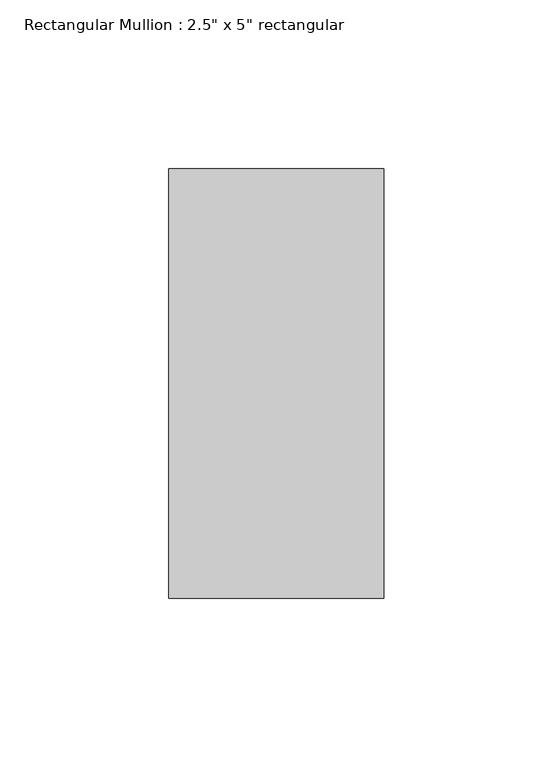
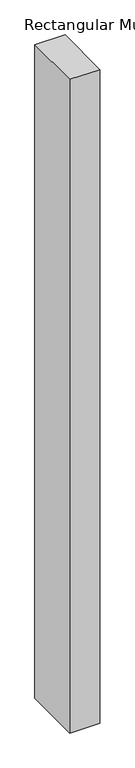
"""IFC4 building model written with IfcOpenShell, lengths in millimetres: member geometry."""

from ifc_helpers import new_model, si_unit, frame, origin, place, context, project, spatial, polyline, outline, extrude, source, transform, mapped, element, save


def member_a6b28368(model_context):
    return source(origin(), model_context, "Body", "SweptSolid", [
        extrude(outline(polyline([(0.0, 63.5), (0.0, -63.5), (-63.5, -63.5), (-63.5, 63.5), (0.0, 63.5)])), frame((0.0, 0.0, -1455.0188321), z_axis=(0.0, 0.0, 1.0), x_axis=(1.0, 0.0, 0.0)), (0.0, 0.0, 1.0), 1455.0188321),
    ])


if __name__ == "__main__":
    model = new_model("IFC4")
    model_context = context("Model", 3, world=origin())
    ifc_project = project(units=[si_unit("LENGTHUNIT", "METRE", prefix="MILLI")], contexts=[model_context])
    site = spatial("IfcSite", under=ifc_project)
    building = spatial("IfcBuilding", under=site)
    placement = place(None, origin())
    member_shape = member_a6b28368(model_context)
    element("IfcMember", 1, ObjectType="Rectangular Mullion : 2.5\" x 5\" rectangular", at=placement, inside=building, context=model_context, shape_type="MappedRepresentation", body=[
        mapped(member_shape, transform((0.0, 0.0, 0.0), x_axis=(1.0, 0.0, 0.0), y_axis=(0.0, 1.0, 0.0), z_axis=(0.0, 0.0, 1.0))),
    ])
    save(model, "model.ifc")

# Revit data of these elements
# Type "Rectangular Mullion : 2.5\" x 5\" rectangular"
#   built-in parameter 1007304 = 0.416667 (stored number, unit not read)
#   built-in parameter 1007301 = 0.104167 (stored number, unit not read)
#   built-in parameter 1007300 = 0.104167 (stored number, unit not read)
# Element 1 (IfcMember, "Rectangular Mullion : 2.5\" x 5\" rectangular")
#   Materials on its faces: "Aluminum"
# Materials
#   "Aluminum": class "Metal", colour RGB 247 247 247, transparency 0, Description = "Aluminum 6061", Cost = 0
